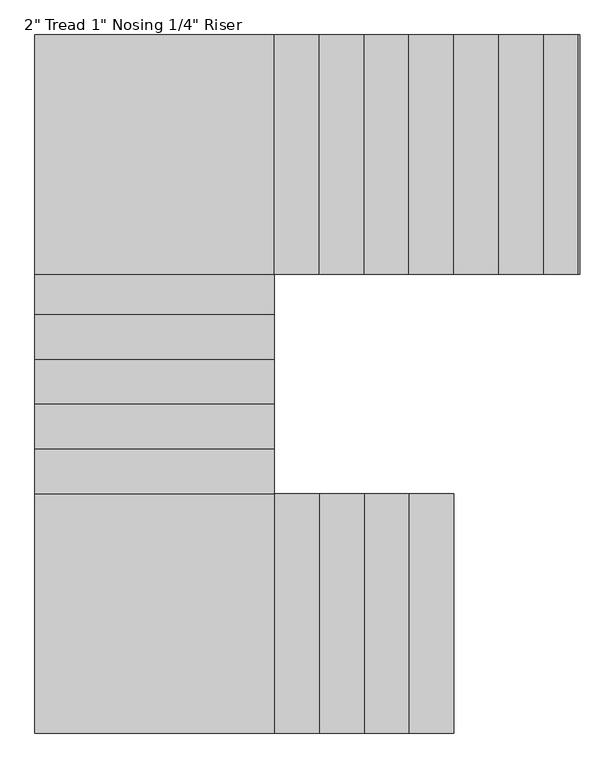
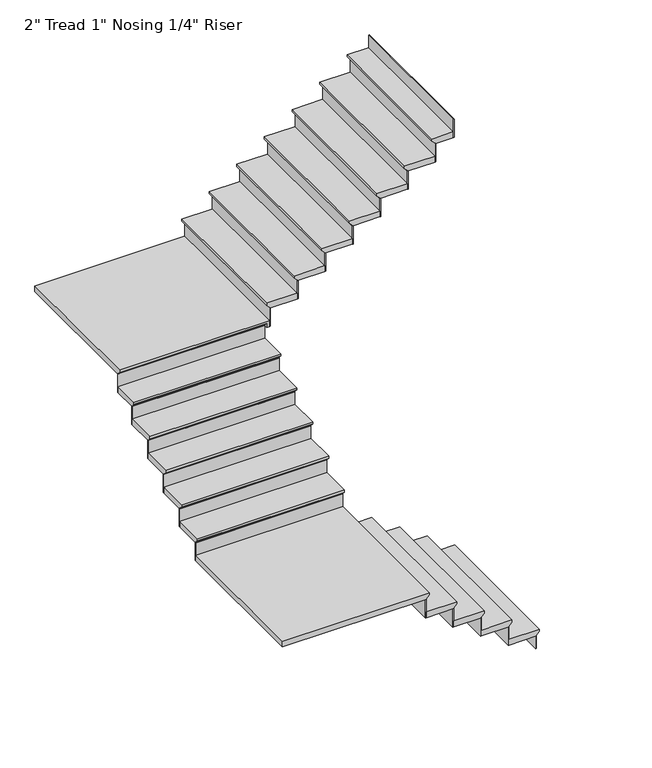
"""IFC4 building model written with IfcOpenShell, lengths in millimetres: stair flight geometry."""

from ifc_helpers import new_model, si_unit, origin, place, context, project, spatial, faceted_brep, source, transform, mapped, element, save


def stair_flight_8c9b7ea6(model_context):
    return source(origin(), model_context, "Body", "Brep", [
        faceted_brep([(-2683.1105391, -1521.8373761, 15990.9710526), (-2683.1105391, -1521.8373761, 16010.0210526), (-2683.1105391, -2741.0373761, 16010.0210526), (-2683.1105391, -2741.0373761, 15990.9710526), (-2708.5105391, -1521.8373761, 15965.5710526), (-2708.5105391, -2741.0373761, 15965.5710526), (-2937.1105391, -1521.8373761, 16010.0210526), (-2937.1105391, -2741.0373761, 16010.0210526), (-2708.5105391, -2741.0373761, 15959.2210526), (-2937.1105391, -2741.0373761, 15959.2210526), (-2937.1105391, -1521.8373761, 15959.2210526), (-2708.5105391, -1521.8373761, 15959.2210526)], [[[0, 1, 2, 3]], [[4, 0, 3, 5]], [[2, 1, 6, 7]], [[8, 9, 10, 11]], [[2, 7, 9, 8, 5, 3]], [[8, 11, 4, 5]], [[6, 1, 0, 4, 11, 10]], [[7, 6, 10, 9]]]),
        faceted_brep([(-2708.5105391, -1521.8373761, 15959.2210526), (-2708.5105391, -1521.8373761, 15849.6), (-2714.8605391, -1521.8373761, 15849.6), (-2714.8605391, -1521.8373761, 15959.2210526), (-2708.5105391, -2741.0373761, 15959.2210526), (-2714.8605391, -2741.0373761, 15959.2210526), (-2714.8605391, -2741.0373761, 15849.6), (-2708.5105391, -2741.0373761, 15849.6)], [[[0, 1, 2, 3]], [[4, 5, 6, 7]], [[1, 0, 4, 7]], [[2, 1, 7, 6]], [[3, 2, 6, 5]], [[0, 3, 5, 4]]]),
        faceted_brep([(-2937.1105391, -1521.8373761, 16119.6421053), (-2937.1105391, -1521.8373761, 15959.2210526), (-2943.4605391, -1521.8373761, 15959.2210526), (-2943.4605391, -1521.8373761, 16119.6421053), (-2937.1105391, -2741.0373761, 16119.6421053), (-2943.4605391, -2741.0373761, 16119.6421053), (-2943.4605391, -2741.0373761, 15959.2210526), (-2937.1105391, -2741.0373761, 15959.2210526)], [[[0, 1, 2, 3]], [[4, 5, 6, 7]], [[1, 0, 4, 7]], [[2, 1, 7, 6]], [[3, 2, 6, 5]], [[0, 3, 5, 4]]]),
        faceted_brep([(-2911.7105391, -2741.0373761, 16170.4421053), (-2911.7105391, -1521.8373761, 16170.4421053), (-3165.7105391, -1521.8373761, 16170.4421053), (-3165.7105391, -2741.0373761, 16170.4421053), (-2937.1105391, -2741.0373761, 16119.6421053), (-3165.7105391, -2741.0373761, 16119.6421053), (-3165.7105391, -1521.8373761, 16119.6421053), (-2937.1105391, -1521.8373761, 16119.6421053), (-2937.1105391, -2741.0373761, 16125.9921053), (-2911.7105391, -2741.0373761, 16151.3921053), (-2937.1105391, -1521.8373761, 16125.9921053), (-2911.7105391, -1521.8373761, 16151.3921053)], [[[0, 1, 2, 3]], [[4, 5, 6, 7]], [[0, 3, 5, 4, 8, 9]], [[4, 7, 10, 8]], [[2, 1, 11, 10, 7, 6]], [[3, 2, 6, 5]], [[11, 1, 0, 9]], [[10, 11, 9, 8]]]),
        faceted_brep([(-3165.7105391, -1521.8373761, 16280.0631579), (-3165.7105391, -1521.8373761, 16119.6421053), (-3172.0605391, -1521.8373761, 16119.6421053), (-3172.0605391, -1521.8373761, 16280.0631579), (-3165.7105391, -2741.0373761, 16280.0631579), (-3172.0605391, -2741.0373761, 16280.0631579), (-3172.0605391, -2741.0373761, 16119.6421053), (-3165.7105391, -2741.0373761, 16119.6421053)], [[[0, 1, 2, 3]], [[4, 5, 6, 7]], [[1, 0, 4, 7]], [[2, 1, 7, 6]], [[3, 2, 6, 5]], [[0, 3, 5, 4]]]),
        faceted_brep([(-3140.3105391, -2741.0373761, 16330.8631579), (-3140.3105391, -1521.8373761, 16330.8631579), (-3394.3105391, -1521.8373761, 16330.8631579), (-3394.3105391, -2741.0373761, 16330.8631579), (-3165.7105391, -2741.0373761, 16280.0631579), (-3394.3105391, -2741.0373761, 16280.0631579), (-3394.3105391, -1521.8373761, 16280.0631579), (-3165.7105391, -1521.8373761, 16280.0631579), (-3165.7105391, -2741.0373761, 16286.4131579), (-3140.3105391, -2741.0373761, 16311.8131579), (-3165.7105391, -1521.8373761, 16286.4131579), (-3140.3105391, -1521.8373761, 16311.8131579)], [[[0, 1, 2, 3]], [[4, 5, 6, 7]], [[0, 3, 5, 4, 8, 9]], [[4, 7, 10, 8]], [[2, 1, 11, 10, 7, 6]], [[3, 2, 6, 5]], [[11, 1, 0, 9]], [[10, 11, 9, 8]]]),
        faceted_brep([(-3394.3105391, -1521.8373761, 16440.4842105), (-3394.3105391, -1521.8373761, 16280.0631579), (-3400.6605391, -1521.8373761, 16280.0631579), (-3400.6605391, -1521.8373761, 16440.4842105), (-3394.3105391, -2741.0373761, 16440.4842105), (-3400.6605391, -2741.0373761, 16440.4842105), (-3400.6605391, -2741.0373761, 16280.0631579), (-3394.3105391, -2741.0373761, 16280.0631579)], [[[0, 1, 2, 3]], [[4, 5, 6, 7]], [[1, 0, 4, 7]], [[2, 1, 7, 6]], [[3, 2, 6, 5]], [[0, 3, 5, 4]]]),
        faceted_brep([(-3368.9105391, -2741.0373761, 16491.2842105), (-3368.9105391, -1521.8373761, 16491.2842105), (-3622.9105391, -1521.8373761, 16491.2842105), (-3622.9105391, -2741.0373761, 16491.2842105), (-3394.3105391, -2741.0373761, 16440.4842105), (-3622.9105391, -2741.0373761, 16440.4842105), (-3622.9105391, -1521.8373761, 16440.4842105), (-3394.3105391, -1521.8373761, 16440.4842105), (-3394.3105391, -2741.0373761, 16446.8342105), (-3368.9105391, -2741.0373761, 16472.2342105), (-3394.3105391, -1521.8373761, 16446.8342105), (-3368.9105391, -1521.8373761, 16472.2342105)], [[[0, 1, 2, 3]], [[4, 5, 6, 7]], [[0, 3, 5, 4, 8, 9]], [[4, 7, 10, 8]], [[2, 1, 11, 10, 7, 6]], [[3, 2, 6, 5]], [[11, 1, 0, 9]], [[10, 11, 9, 8]]]),
        faceted_brep([(-3622.9105391, -1521.8373761, 16600.9052632), (-3622.9105391, -1521.8373761, 16440.4842105), (-3629.2605391, -1521.8373761, 16440.4842105), (-3629.2605391, -1521.8373761, 16600.9052632), (-3622.9105391, -2741.0373761, 16600.9052632), (-3629.2605391, -2741.0373761, 16600.9052632), (-3629.2605391, -2741.0373761, 16440.4842105), (-3622.9105391, -2741.0373761, 16440.4842105)], [[[0, 1, 2, 3]], [[4, 5, 6, 7]], [[1, 0, 4, 7]], [[2, 1, 7, 6]], [[3, 2, 6, 5]], [[0, 3, 5, 4]]]),
        faceted_brep([(-4816.7105391, -1496.4373761, 16651.7052632), (-4816.7105391, -2741.0373761, 16651.7052632), (-3597.5105391, -2741.0373761, 16651.7052632), (-3597.5105391, -1496.4373761, 16651.7052632), (-4816.7105391, -2741.0373761, 16600.9052632), (-4816.7105391, -1496.4373761, 16600.9052632), (-3597.5105391, -1496.4373761, 16600.9052632), (-3597.5105391, -1521.8373761, 16600.9052632), (-3622.9105391, -1521.8373761, 16600.9052632), (-3622.9105391, -2741.0373761, 16600.9052632), (-3622.9105391, -2741.0373761, 16607.2552632), (-3597.5105391, -2741.0373761, 16632.6552632), (-3622.9105391, -1521.8373761, 16607.2552632), (-3597.5105391, -1521.8373761, 16632.6552632)], [[[0, 1, 2, 3]], [[4, 5, 6, 7, 8, 9]], [[1, 0, 5, 4]], [[2, 1, 4, 9, 10, 11]], [[9, 8, 12, 10]], [[8, 7, 13, 12]], [[3, 2, 11, 13, 7, 6]], [[0, 3, 6, 5]], [[11, 10, 12, 13]]]),
        faceted_brep([(-3597.5105391, -1496.4373761, 16761.3263158), (-3597.5105391, -1496.4373761, 16600.9052632), (-3597.5105391, -1490.0873761, 16600.9052632), (-3597.5105391, -1490.0873761, 16761.3263158), (-4816.7105391, -1496.4373761, 16761.3263158), (-4816.7105391, -1490.0873761, 16761.3263158), (-4816.7105391, -1490.0873761, 16600.9052632), (-4816.7105391, -1496.4373761, 16600.9052632)], [[[0, 1, 2, 3]], [[4, 5, 6, 7]], [[1, 0, 4, 7]], [[2, 1, 7, 6]], [[3, 2, 6, 5]], [[0, 3, 5, 4]]]),
        faceted_brep([(-4816.7105391, -1521.8373761, 16812.1263158), (-3597.5105391, -1521.8373761, 16812.1263158), (-3597.5105391, -1267.8373761, 16812.1263158), (-4816.7105391, -1267.8373761, 16812.1263158), (-4816.7105391, -1496.4373761, 16761.3263158), (-4816.7105391, -1267.8373761, 16761.3263158), (-3597.5105391, -1267.8373761, 16761.3263158), (-3597.5105391, -1496.4373761, 16761.3263158), (-4816.7105391, -1496.4373761, 16767.6763158), (-4816.7105391, -1521.8373761, 16793.0763158), (-3597.5105391, -1496.4373761, 16767.6763158), (-3597.5105391, -1521.8373761, 16793.0763158)], [[[0, 1, 2, 3]], [[4, 5, 6, 7]], [[0, 3, 5, 4, 8, 9]], [[4, 7, 10, 8]], [[2, 1, 11, 10, 7, 6]], [[3, 2, 6, 5]], [[11, 1, 0, 9]], [[10, 11, 9, 8]]]),
        faceted_brep([(-3597.5105391, -1267.8373761, 16921.7473684), (-3597.5105391, -1267.8373761, 16761.3263158), (-3597.5105391, -1261.4873761, 16761.3263158), (-3597.5105391, -1261.4873761, 16921.7473684), (-4816.7105391, -1267.8373761, 16921.7473684), (-4816.7105391, -1261.4873761, 16921.7473684), (-4816.7105391, -1261.4873761, 16761.3263158), (-4816.7105391, -1267.8373761, 16761.3263158)], [[[0, 1, 2, 3]], [[4, 5, 6, 7]], [[1, 0, 4, 7]], [[2, 1, 7, 6]], [[3, 2, 6, 5]], [[0, 3, 5, 4]]]),
        faceted_brep([(-4816.7105391, -1293.2373761, 16972.5473684), (-3597.5105391, -1293.2373761, 16972.5473684), (-3597.5105391, -1039.2373761, 16972.5473684), (-4816.7105391, -1039.2373761, 16972.5473684), (-4816.7105391, -1267.8373761, 16921.7473684), (-4816.7105391, -1039.2373761, 16921.7473684), (-3597.5105391, -1039.2373761, 16921.7473684), (-3597.5105391, -1267.8373761, 16921.7473684), (-4816.7105391, -1267.8373761, 16928.0973684), (-4816.7105391, -1293.2373761, 16953.4973684), (-3597.5105391, -1267.8373761, 16928.0973684), (-3597.5105391, -1293.2373761, 16953.4973684)], [[[0, 1, 2, 3]], [[4, 5, 6, 7]], [[0, 3, 5, 4, 8, 9]], [[4, 7, 10, 8]], [[2, 1, 11, 10, 7, 6]], [[3, 2, 6, 5]], [[11, 1, 0, 9]], [[10, 11, 9, 8]]]),
        faceted_brep([(-3597.5105391, -1039.2373761, 17082.1684211), (-3597.5105391, -1039.2373761, 16921.7473684), (-3597.5105391, -1032.8873761, 16921.7473684), (-3597.5105391, -1032.8873761, 17082.1684211), (-4816.7105391, -1039.2373761, 17082.1684211), (-4816.7105391, -1032.8873761, 17082.1684211), (-4816.7105391, -1032.8873761, 16921.7473684), (-4816.7105391, -1039.2373761, 16921.7473684)], [[[0, 1, 2, 3]], [[4, 5, 6, 7]], [[1, 0, 4, 7]], [[2, 1, 7, 6]], [[3, 2, 6, 5]], [[0, 3, 5, 4]]]),
        faceted_brep([(-4816.7105391, -1064.6373761, 17132.9684211), (-3597.5105391, -1064.6373761, 17132.9684211), (-3597.5105391, -810.6373761, 17132.9684211), (-4816.7105391, -810.6373761, 17132.9684211), (-4816.7105391, -1039.2373761, 17082.1684211), (-4816.7105391, -810.6373761, 17082.1684211), (-3597.5105391, -810.6373761, 17082.1684211), (-3597.5105391, -1039.2373761, 17082.1684211), (-4816.7105391, -1039.2373761, 17088.5184211), (-4816.7105391, -1064.6373761, 17113.9184211), (-3597.5105391, -1039.2373761, 17088.5184211), (-3597.5105391, -1064.6373761, 17113.9184211)], [[[0, 1, 2, 3]], [[4, 5, 6, 7]], [[0, 3, 5, 4, 8, 9]], [[4, 7, 10, 8]], [[2, 1, 11, 10, 7, 6]], [[3, 2, 6, 5]], [[11, 1, 0, 9]], [[10, 11, 9, 8]]]),
        faceted_brep([(-3597.5105391, -810.6373761, 17242.5894737), (-3597.5105391, -810.6373761, 17082.1684211), (-3597.5105391, -804.2873761, 17082.1684211), (-3597.5105391, -804.2873761, 17242.5894737), (-4816.7105391, -810.6373761, 17242.5894737), (-4816.7105391, -804.2873761, 17242.5894737), (-4816.7105391, -804.2873761, 17082.1684211), (-4816.7105391, -810.6373761, 17082.1684211)], [[[0, 1, 2, 3]], [[4, 5, 6, 7]], [[1, 0, 4, 7]], [[2, 1, 7, 6]], [[3, 2, 6, 5]], [[0, 3, 5, 4]]]),
        faceted_brep([(-4816.7105391, -836.0373761, 17293.3894737), (-3597.5105391, -836.0373761, 17293.3894737), (-3597.5105391, -582.0373761, 17293.3894737), (-4816.7105391, -582.0373761, 17293.3894737), (-4816.7105391, -810.6373761, 17242.5894737), (-4816.7105391, -582.0373761, 17242.5894737), (-3597.5105391, -582.0373761, 17242.5894737), (-3597.5105391, -810.6373761, 17242.5894737), (-4816.7105391, -810.6373761, 17248.9394737), (-4816.7105391, -836.0373761, 17274.3394737), (-3597.5105391, -810.6373761, 17248.9394737), (-3597.5105391, -836.0373761, 17274.3394737)], [[[0, 1, 2, 3]], [[4, 5, 6, 7]], [[0, 3, 5, 4, 8, 9]], [[4, 7, 10, 8]], [[2, 1, 11, 10, 7, 6]], [[3, 2, 6, 5]], [[11, 1, 0, 9]], [[10, 11, 9, 8]]]),
        faceted_brep([(-3597.5105391, -582.0373761, 17403.0105263), (-3597.5105391, -582.0373761, 17242.5894737), (-3597.5105391, -575.6873761, 17242.5894737), (-3597.5105391, -575.6873761, 17403.0105263), (-4816.7105391, -582.0373761, 17403.0105263), (-4816.7105391, -575.6873761, 17403.0105263), (-4816.7105391, -575.6873761, 17242.5894737), (-4816.7105391, -582.0373761, 17242.5894737)], [[[0, 1, 2, 3]], [[4, 5, 6, 7]], [[1, 0, 4, 7]], [[2, 1, 7, 6]], [[3, 2, 6, 5]], [[0, 3, 5, 4]]]),
        faceted_brep([(-4816.7105391, -607.4373761, 17453.8105263), (-3597.5105391, -607.4373761, 17453.8105263), (-3597.5105391, -378.8373761, 17453.8105263), (-4816.7105391, -378.8373761, 17453.8105263), (-4816.7105391, -582.0373761, 17403.0105263), (-4816.7105391, -378.8373761, 17403.0105263), (-3597.5105391, -378.8373761, 17403.0105263), (-3597.5105391, -582.0373761, 17403.0105263), (-4816.7105391, -582.0373761, 17409.3605263), (-4816.7105391, -607.4373761, 17434.7605263), (-3597.5105391, -582.0373761, 17409.3605263), (-3597.5105391, -607.4373761, 17434.7605263)], [[[0, 1, 2, 3]], [[4, 5, 6, 7]], [[0, 3, 5, 4, 8, 9]], [[4, 7, 10, 8]], [[2, 1, 11, 10, 7, 6]], [[3, 2, 6, 5]], [[11, 1, 0, 9]], [[10, 11, 9, 8]]]),
        faceted_brep([(-3597.5105391, -378.8373761, 17563.4315789), (-3597.5105391, -378.8373761, 17403.0105263), (-3597.5105391, -372.4873761, 17403.0105263), (-3597.5105391, -372.4873761, 17563.4315789), (-4816.7105391, -378.8373761, 17563.4315789), (-4816.7105391, -372.4873761, 17563.4315789), (-4816.7105391, -372.4873761, 17403.0105263), (-4816.7105391, -378.8373761, 17403.0105263)], [[[0, 1, 2, 3]], [[4, 5, 6, 7]], [[1, 0, 4, 7]], [[2, 1, 7, 6]], [[3, 2, 6, 5]], [[0, 3, 5, 4]]]),
        faceted_brep([(-3572.1105391, 814.9626239, 17614.2315789), (-4816.7105391, 814.9626239, 17614.2315789), (-4816.7105391, -404.2373761, 17614.2315789), (-3572.1105391, -404.2373761, 17614.2315789), (-4816.7105391, 814.9626239, 17563.4315789), (-3572.1105391, 814.9626239, 17563.4315789), (-3572.1105391, -404.2373761, 17563.4315789), (-3597.5105391, -404.2373761, 17563.4315789), (-3597.5105391, -378.8373761, 17563.4315789), (-4816.7105391, -378.8373761, 17563.4315789), (-4816.7105391, -378.8373761, 17569.7815789), (-4816.7105391, -404.2373761, 17595.1815789), (-3597.5105391, -378.8373761, 17569.7815789), (-3597.5105391, -404.2373761, 17595.1815789)], [[[0, 1, 2, 3]], [[4, 5, 6, 7, 8, 9]], [[1, 0, 5, 4]], [[2, 1, 4, 9, 10, 11]], [[9, 8, 12, 10]], [[8, 7, 13, 12]], [[3, 2, 11, 13, 7, 6]], [[0, 3, 6, 5]], [[11, 10, 12, 13]]]),
        faceted_brep([(-3572.1105391, -404.2373761, 17723.8526316), (-3572.1105391, -404.2373761, 17563.4315789), (-3565.7605391, -404.2373761, 17563.4315789), (-3565.7605391, -404.2373761, 17723.8526316), (-3572.1105391, 814.9626239, 17723.8526316), (-3565.7605391, 814.9626239, 17723.8526316), (-3565.7605391, 814.9626239, 17563.4315789), (-3572.1105391, 814.9626239, 17563.4315789)], [[[0, 1, 2, 3]], [[4, 5, 6, 7]], [[1, 0, 4, 7]], [[2, 1, 7, 6]], [[3, 2, 6, 5]], [[0, 3, 5, 4]]]),
        faceted_brep([(-3597.5105391, 814.9626239, 17774.6526316), (-3597.5105391, -404.2373761, 17774.6526316), (-3343.5105391, -404.2373761, 17774.6526316), (-3343.5105391, 814.9626239, 17774.6526316), (-3572.1105391, 814.9626239, 17723.8526316), (-3343.5105391, 814.9626239, 17723.8526316), (-3343.5105391, -404.2373761, 17723.8526316), (-3572.1105391, -404.2373761, 17723.8526316), (-3572.1105391, 814.9626239, 17730.2026316), (-3597.5105391, 814.9626239, 17755.6026316), (-3572.1105391, -404.2373761, 17730.2026316), (-3597.5105391, -404.2373761, 17755.6026316)], [[[0, 1, 2, 3]], [[4, 5, 6, 7]], [[0, 3, 5, 4, 8, 9]], [[4, 7, 10, 8]], [[2, 1, 11, 10, 7, 6]], [[3, 2, 6, 5]], [[11, 1, 0, 9]], [[10, 11, 9, 8]]]),
        faceted_brep([(-3343.5105391, -404.2373761, 17884.2736842), (-3343.5105391, -404.2373761, 17723.8526316), (-3337.1605391, -404.2373761, 17723.8526316), (-3337.1605391, -404.2373761, 17884.2736842), (-3343.5105391, 814.9626239, 17884.2736842), (-3337.1605391, 814.9626239, 17884.2736842), (-3337.1605391, 814.9626239, 17723.8526316), (-3343.5105391, 814.9626239, 17723.8526316)], [[[0, 1, 2, 3]], [[4, 5, 6, 7]], [[1, 0, 4, 7]], [[2, 1, 7, 6]], [[3, 2, 6, 5]], [[0, 3, 5, 4]]]),
        faceted_brep([(-3368.9105391, 814.9626239, 17935.0736842), (-3368.9105391, -404.2373761, 17935.0736842), (-3114.9105391, -404.2373761, 17935.0736842), (-3114.9105391, 814.9626239, 17935.0736842), (-3343.5105391, 814.9626239, 17884.2736842), (-3114.9105391, 814.9626239, 17884.2736842), (-3114.9105391, -404.2373761, 17884.2736842), (-3343.5105391, -404.2373761, 17884.2736842), (-3343.5105391, 814.9626239, 17890.6236842), (-3368.9105391, 814.9626239, 17916.0236842), (-3343.5105391, -404.2373761, 17890.6236842), (-3368.9105391, -404.2373761, 17916.0236842)], [[[0, 1, 2, 3]], [[4, 5, 6, 7]], [[0, 3, 5, 4, 8, 9]], [[4, 7, 10, 8]], [[2, 1, 11, 10, 7, 6]], [[3, 2, 6, 5]], [[11, 1, 0, 9]], [[10, 11, 9, 8]]]),
        faceted_brep([(-3114.9105391, -404.2373761, 18044.6947368), (-3114.9105391, -404.2373761, 17884.2736842), (-3108.5605391, -404.2373761, 17884.2736842), (-3108.5605391, -404.2373761, 18044.6947368), (-3114.9105391, 814.9626239, 18044.6947368), (-3108.5605391, 814.9626239, 18044.6947368), (-3108.5605391, 814.9626239, 17884.2736842), (-3114.9105391, 814.9626239, 17884.2736842)], [[[0, 1, 2, 3]], [[4, 5, 6, 7]], [[1, 0, 4, 7]], [[2, 1, 7, 6]], [[3, 2, 6, 5]], [[0, 3, 5, 4]]]),
        faceted_brep([(-3140.3105391, 814.9626239, 18095.4947368), (-3140.3105391, -404.2373761, 18095.4947368), (-2886.3105391, -404.2373761, 18095.4947368), (-2886.3105391, 814.9626239, 18095.4947368), (-3114.9105391, 814.9626239, 18044.6947368), (-2886.3105391, 814.9626239, 18044.6947368), (-2886.3105391, -404.2373761, 18044.6947368), (-3114.9105391, -404.2373761, 18044.6947368), (-3114.9105391, 814.9626239, 18051.0447368), (-3140.3105391, 814.9626239, 18076.4447368), (-3114.9105391, -404.2373761, 18051.0447368), (-3140.3105391, -404.2373761, 18076.4447368)], [[[0, 1, 2, 3]], [[4, 5, 6, 7]], [[0, 3, 5, 4, 8, 9]], [[4, 7, 10, 8]], [[2, 1, 11, 10, 7, 6]], [[3, 2, 6, 5]], [[11, 1, 0, 9]], [[10, 11, 9, 8]]]),
        faceted_brep([(-2886.3105391, -404.2373761, 18205.1157895), (-2886.3105391, -404.2373761, 18044.6947368), (-2879.9605391, -404.2373761, 18044.6947368), (-2879.9605391, -404.2373761, 18205.1157895), (-2886.3105391, 814.9626239, 18205.1157895), (-2879.9605391, 814.9626239, 18205.1157895), (-2879.9605391, 814.9626239, 18044.6947368), (-2886.3105391, 814.9626239, 18044.6947368)], [[[0, 1, 2, 3]], [[4, 5, 6, 7]], [[1, 0, 4, 7]], [[2, 1, 7, 6]], [[3, 2, 6, 5]], [[0, 3, 5, 4]]]),
        faceted_brep([(-2911.7105391, 814.9626239, 18255.9157895), (-2911.7105391, -404.2373761, 18255.9157895), (-2657.7105391, -404.2373761, 18255.9157895), (-2657.7105391, 814.9626239, 18255.9157895), (-2886.3105391, 814.9626239, 18205.1157895), (-2657.7105391, 814.9626239, 18205.1157895), (-2657.7105391, -404.2373761, 18205.1157895), (-2886.3105391, -404.2373761, 18205.1157895), (-2886.3105391, 814.9626239, 18211.4657895), (-2911.7105391, 814.9626239, 18236.8657895), (-2886.3105391, -404.2373761, 18211.4657895), (-2911.7105391, -404.2373761, 18236.8657895)], [[[0, 1, 2, 3]], [[4, 5, 6, 7]], [[0, 3, 5, 4, 8, 9]], [[4, 7, 10, 8]], [[2, 1, 11, 10, 7, 6]], [[3, 2, 6, 5]], [[11, 1, 0, 9]], [[10, 11, 9, 8]]]),
        faceted_brep([(-2657.7105391, -404.2373761, 18365.5368421), (-2657.7105391, -404.2373761, 18205.1157895), (-2651.3605391, -404.2373761, 18205.1157895), (-2651.3605391, -404.2373761, 18365.5368421), (-2657.7105391, 814.9626239, 18365.5368421), (-2651.3605391, 814.9626239, 18365.5368421), (-2651.3605391, 814.9626239, 18205.1157895), (-2657.7105391, 814.9626239, 18205.1157895)], [[[0, 1, 2, 3]], [[4, 5, 6, 7]], [[1, 0, 4, 7]], [[2, 1, 7, 6]], [[3, 2, 6, 5]], [[0, 3, 5, 4]]]),
        faceted_brep([(-2683.1105391, 814.9626239, 18416.3368421), (-2683.1105391, -404.2373761, 18416.3368421), (-2429.1105391, -404.2373761, 18416.3368421), (-2429.1105391, 814.9626239, 18416.3368421), (-2657.7105391, 814.9626239, 18365.5368421), (-2429.1105391, 814.9626239, 18365.5368421), (-2429.1105391, -404.2373761, 18365.5368421), (-2657.7105391, -404.2373761, 18365.5368421), (-2657.7105391, 814.9626239, 18371.8868421), (-2683.1105391, 814.9626239, 18397.2868421), (-2657.7105391, -404.2373761, 18371.8868421), (-2683.1105391, -404.2373761, 18397.2868421)], [[[0, 1, 2, 3]], [[4, 5, 6, 7]], [[0, 3, 5, 4, 8, 9]], [[4, 7, 10, 8]], [[2, 1, 11, 10, 7, 6]], [[3, 2, 6, 5]], [[11, 1, 0, 9]], [[10, 11, 9, 8]]]),
        faceted_brep([(-2429.1105391, -404.2373761, 18525.9578947), (-2429.1105391, -404.2373761, 18365.5368421), (-2422.7605391, -404.2373761, 18365.5368421), (-2422.7605391, -404.2373761, 18525.9578947), (-2429.1105391, 814.9626239, 18525.9578947), (-2422.7605391, 814.9626239, 18525.9578947), (-2422.7605391, 814.9626239, 18365.5368421), (-2429.1105391, 814.9626239, 18365.5368421)], [[[0, 1, 2, 3]], [[4, 5, 6, 7]], [[1, 0, 4, 7]], [[2, 1, 7, 6]], [[3, 2, 6, 5]], [[0, 3, 5, 4]]]),
        faceted_brep([(-2454.5105391, 814.9626239, 18576.7578947), (-2454.5105391, -404.2373761, 18576.7578947), (-2200.5105391, -404.2373761, 18576.7578947), (-2200.5105391, 814.9626239, 18576.7578947), (-2429.1105391, 814.9626239, 18525.9578947), (-2200.5105391, 814.9626239, 18525.9578947), (-2200.5105391, -404.2373761, 18525.9578947), (-2429.1105391, -404.2373761, 18525.9578947), (-2429.1105391, 814.9626239, 18532.3078947), (-2454.5105391, 814.9626239, 18557.7078947), (-2429.1105391, -404.2373761, 18532.3078947), (-2454.5105391, -404.2373761, 18557.7078947)], [[[0, 1, 2, 3]], [[4, 5, 6, 7]], [[0, 3, 5, 4, 8, 9]], [[4, 7, 10, 8]], [[2, 1, 11, 10, 7, 6]], [[3, 2, 6, 5]], [[11, 1, 0, 9]], [[10, 11, 9, 8]]]),
        faceted_brep([(-2200.5105391, -404.2373761, 18686.3789474), (-2200.5105391, -404.2373761, 18525.9578947), (-2194.1605391, -404.2373761, 18525.9578947), (-2194.1605391, -404.2373761, 18686.3789474), (-2200.5105391, 814.9626239, 18686.3789474), (-2194.1605391, 814.9626239, 18686.3789474), (-2194.1605391, 814.9626239, 18525.9578947), (-2200.5105391, 814.9626239, 18525.9578947)], [[[0, 1, 2, 3]], [[4, 5, 6, 7]], [[1, 0, 4, 7]], [[2, 1, 7, 6]], [[3, 2, 6, 5]], [[0, 3, 5, 4]]]),
        faceted_brep([(-2048.1105391, -404.2373761, 18846.8), (-2048.1105391, -404.2373761, 18686.3789474), (-2041.7605391, -404.2373761, 18686.3789474), (-2041.7605391, -404.2373761, 18846.8), (-2048.1105391, 814.9626239, 18846.8), (-2041.7605391, 814.9626239, 18846.8), (-2041.7605391, 814.9626239, 18686.3789474), (-2048.1105391, 814.9626239, 18686.3789474)], [[[0, 1, 2, 3]], [[4, 5, 6, 7]], [[1, 0, 4, 7]], [[2, 1, 7, 6]], [[3, 2, 6, 5]], [[0, 3, 5, 4]]]),
        faceted_brep([(-2225.9105391, 814.9626239, 18737.1789474), (-2225.9105391, -404.2373761, 18737.1789474), (-2048.1105391, -404.2373761, 18737.1789474), (-2048.1105391, 814.9626239, 18737.1789474), (-2200.5105391, 814.9626239, 18686.3789474), (-2048.1105391, 814.9626239, 18686.3789474), (-2048.1105391, -404.2373761, 18686.3789474), (-2200.5105391, -404.2373761, 18686.3789474), (-2200.5105391, 814.9626239, 18692.7289474), (-2225.9105391, 814.9626239, 18718.1289474), (-2200.5105391, -404.2373761, 18692.7289474), (-2225.9105391, -404.2373761, 18718.1289474)], [[[0, 1, 2, 3]], [[4, 5, 6, 7]], [[0, 3, 5, 4, 8, 9]], [[4, 7, 10, 8]], [[2, 1, 11, 10, 7, 6]], [[3, 2, 6, 5]], [[11, 1, 0, 9]], [[10, 11, 9, 8]]]),
    ])


if __name__ == "__main__":
    model = new_model("IFC4")
    model_context = context("Model", 3, world=origin())
    ifc_project = project(units=[si_unit("LENGTHUNIT", "METRE", prefix="MILLI")], contexts=[model_context])
    site = spatial("IfcSite", under=ifc_project)
    building = spatial("IfcBuilding", under=site)
    placement = place(None, origin())
    stair_flight_shape = stair_flight_8c9b7ea6(model_context)
    element("IfcStairFlight", 1, ObjectType="2\" Tread 1\" Nosing 1/4\" Riser", at=placement, inside=building, context=model_context, shape_type="MappedRepresentation", body=[
        mapped(stair_flight_shape, transform((0.0, 0.0, 0.0), x_axis=(1.0, 0.0, 0.0), y_axis=(0.0, 1.0, 0.0), z_axis=(0.0, 0.0, 1.0))),
    ])
    save(model, "model.ifc")
